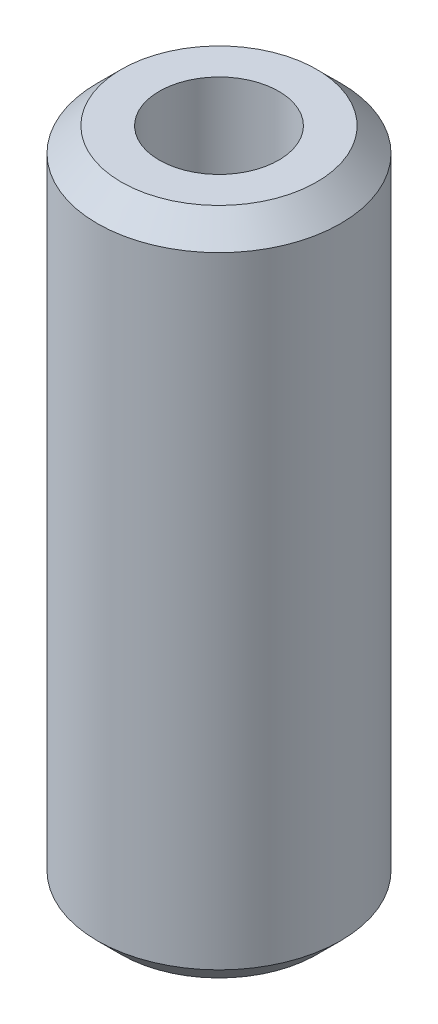
SolidWorks part; units mm, degrees
material "Plain Carbon Steel"
ref_plane "Front Plane" through (0, 0, 0) normal (0, 0, 1) x (1, 0, 0)
ref_plane "Top Plane" through (0, 0, 0) normal (0, 1, 0) x (1, 0, 0)
ref_plane "Right Plane" through (0, 0, 0) normal (1, 0, 0) x (0, 0, -1)
sketch "Pin Profile Ø25.4-Ø12.47" plane through (0, 0, 0) normal (0, 1, 0) x (1, 0, 0)
  circle A0 centre (0, 0) radius 6.235
  circle A1 centre (0, 0) radius 12.7
  dimension "D1" = 12.47
  dimension "D2" = 25.4
extrude "Pin Body 69.85" add sketch "Pin Profile Ø25.4-Ø12.47" along normal mid plane 69.85
chamfer "End Chamfers 2.5x45°" distance 2.5 angle 45 2 edges at (0, -34.925, 12.7) (0, 34.925, 12.7)
